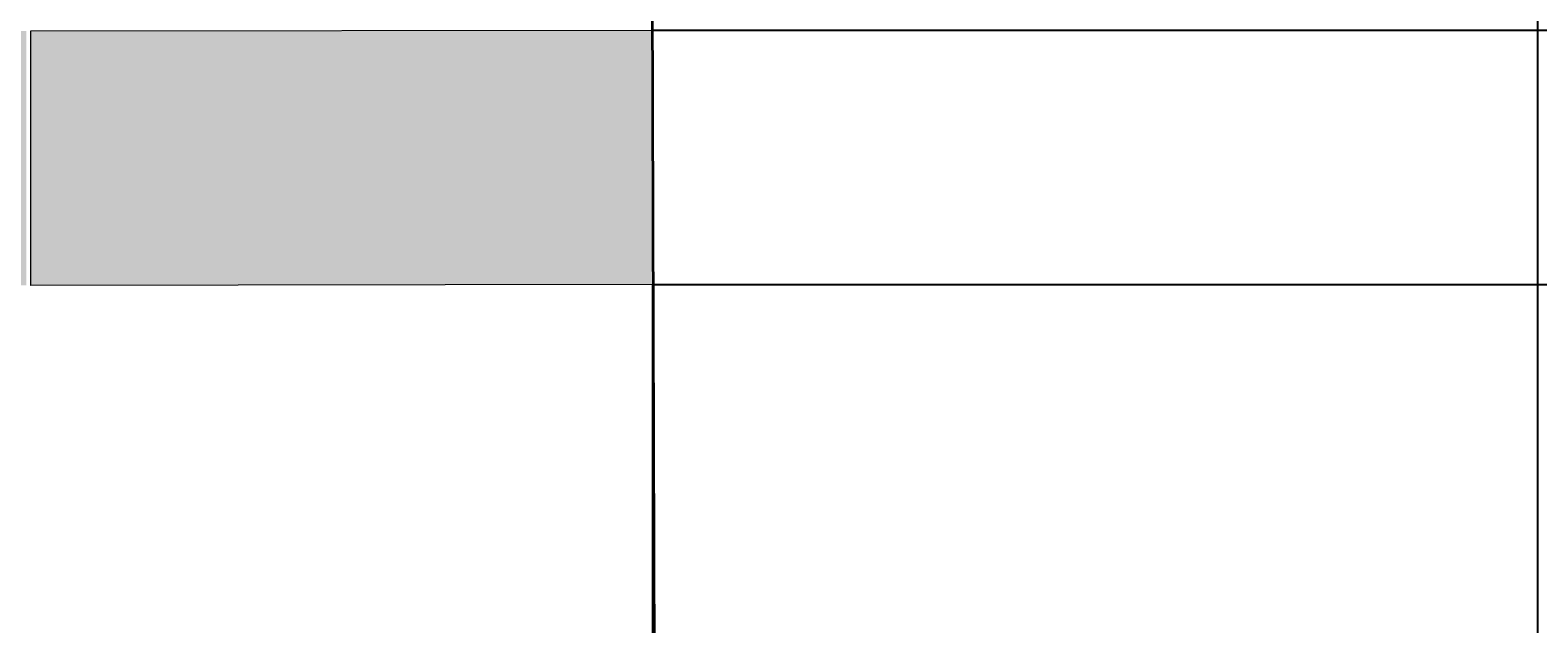
# Model space of a CAD drawing. Units: inches. Extents: x -26 to 776, y -22 to 650.
# Tile 39 of 62: x 309 to 426, y 502 to 548. Entities that reach past the tile are written whole.
import ezdxf

# ---------------------------------------------------------------- set-up
doc = ezdxf.new("R2010")
doc.units = ezdxf.units.IN
doc.header["$MEASUREMENT"] = 0
for name, color, linetype, lineweight in [('A-ANNO-DIMS', 2, 'Continuous', 18), ('A-GLAZ', 4, 'Continuous', 18), ('A-GLAZ-PATT', 9, 'Continuous', 13), ('A-WALL', 7, 'Continuous', 35)]:
    doc.layers.add(name, color=color, linetype=linetype, lineweight=lineweight)
doc.styles.get("Standard").update_dxf_attribs({"font": 'arial.ttf'})
doc.dimstyles.get("Standard").update_dxf_attribs({"dimtxt": 0.5625, "dimasz": 0.18, "dimexe": 0.18, "dimexo": 0.0625, "dimgap": 0.09, "dimtad": 0, "dimtih": 1, "dimtoh": 1, "dimdec": 4, "dimzin": 0, "dimdsep": 46, "dimlunit": 4, "dimtxsty": 'Standard', "dimcen": 0.09, "dimadec": 0, "dimazin": 0, "dimtfac": 1, "dimtdec": 4, "dimtofl": 0, "dimtmove": 0, "dimatfit": 3, "dimfxl": 1, "dimtolj": 1, "dimtzin": 0, "dimarcsym": 0})

# ---------------------------------------------------------------- blocks, each defined once
blk = doc.blocks.new('*D33')
at = {"layer": 'A-ANNO-DIMS', "color": 0, "lineweight": -2, "transparency": 16777216}
for p, q in [((357.37, 548.1), (775.34, 548.1)), ((775.16, 547.92), (775.16, 538.64)), ((775.16, 528.6), (775.16, 537.88)), ((357.37, 528.42), (775.34, 528.42))]:
    blk.add_line(p, q, dxfattribs=at)
at = {"layer": 'A-ANNO-DIMS', "color": 0, "transparency": 16777216}
for points in [[(775.13, 547.92), (775.19, 547.92), (775.16, 548.1)], [(775.13, 528.6), (775.19, 528.6), (775.16, 528.42)]]:
    blk.add_solid(points, dxfattribs=at)
at = {"layer": 'Defpoints', "color": 0, "transparency": 16777216}
for p in [(357.3, 548.1), (775.16, 548.1), (357.3, 528.42)]:
    blk.add_point(p, dxfattribs=at)
at = {"layer": 'A-ANNO-DIMS', "color": 0, "transparency": 16777216, "insert": (775.16, 538.26), "char_height": 0.562, "attachment_point": 5}
blk.add_mtext('\\A1;19.676', dxfattribs=at)
blk = doc.blocks.new('*D34')
at = {"layer": 'A-ANNO-DIMS', "color": 0, "lineweight": -2, "transparency": 16777216}
for p, q in [((228.57, 528.3), (228.57, -21.31)), ((357.3, 528.36), (357.3, -21.31)), ((228.75, -21.13), (291.71, -21.13)), ((357.12, -21.13), (294.17, -21.13))]:
    blk.add_line(p, q, dxfattribs=at)
at = {"layer": 'A-ANNO-DIMS', "color": 0, "transparency": 16777216}
for points in [[(228.75, -21.1), (228.75, -21.16), (228.57, -21.13)], [(357.12, -21.1), (357.12, -21.16), (357.3, -21.13)]]:
    blk.add_solid(points, dxfattribs=at)
at = {"layer": 'Defpoints', "color": 0, "transparency": 16777216}
for p in [(228.57, 528.36), (357.3, 528.42), (357.3, -21.13)]:
    blk.add_point(p, dxfattribs=at)
at = {"layer": 'A-ANNO-DIMS', "color": 0, "transparency": 16777216, "insert": (292.94, -21.13), "char_height": 0.562, "attachment_point": 5}
blk.add_mtext('\\A1;128.73', dxfattribs=at)
blk = doc.blocks.new('*D39')
at = {"layer": 'A-ANNO-DIMS', "color": 0, "lineweight": -2, "transparency": 16777216}
for p, q in [((289.24, 15.54), (289.24, 649.86)), ((289.42, 649.68), (356.48, 649.68)), ((425.56, 649.68), (358.51, 649.68)), ((425.74, 15.54), (425.74, 649.86))]:
    blk.add_line(p, q, dxfattribs=at)
at = {"layer": 'A-ANNO-DIMS', "color": 0, "transparency": 16777216}
for points in [[(289.42, 649.71), (289.42, 649.65), (289.24, 649.68)], [(425.56, 649.71), (425.56, 649.65), (425.74, 649.68)]]:
    blk.add_solid(points, dxfattribs=at)
at = {"layer": 'Defpoints', "color": 0, "transparency": 16777216}
for p in [(425.74, 649.68), (289.24, 15.48), (425.74, 15.48)]:
    blk.add_point(p, dxfattribs=at)
at = {"layer": 'A-ANNO-DIMS', "color": 0, "transparency": 16777216, "insert": (357.49, 649.68), "char_height": 0.562, "attachment_point": 5}
blk.add_mtext('\\A1;136.5', dxfattribs=at)

msp = doc.modelspace()

# ---------------------------------------------------------------- hatches: boundary and pattern name
at = {"layer": 'A-GLAZ-PATT'}
h = msp.add_hatch(dxfattribs=at)
h.set_pattern_fill('GOST_GLASS', color=256, scale=0.75)
h.set_pattern_definition([(45, (0, 0), (6.36396, 0), [3.75, -5.25]), (45, (1.591, 0), (6.36396, 0), [1.5, -7.5]), (45, (0, 1.591), (6.36396, 0), [1.5, -7.5])])
h.paths.add_polyline_path([(115.8402, 198.8773), (93.6448, 198.8773), (93.6448, 173.9734), (115.8402, 173.9734)])
h.paths.add_polyline_path([(144.1571, 198.8773), (115.8402, 198.8773), (115.8402, 173.9734), (144.1571, 173.9734)])
h.paths.add_polyline_path([(115.8402, 224.3396), (93.6448, 224.3396), (93.6448, 198.8773), (115.8402, 198.8773)])
h.paths.add_polyline_path([(144.1571, 248.4417), (115.8402, 248.4417), (115.8402, 224.3396), (144.1571, 224.3396)])
h.paths.add_polyline_path([(144.1571, 224.3396), (115.8402, 224.3396), (115.8402, 198.8773), (144.1571, 198.8773)])
h.paths.add_polyline_path([(170.5449, 224.3396), (144.1571, 224.3396), (144.1571, 198.8773), (170.5449, 198.8773)])
h.paths.add_polyline_path([(170.5449, 198.8773), (144.1571, 198.8773), (144.1571, 173.9734), (170.5449, 173.9734)])
h.paths.add_polyline_path([(194.6694, 198.8773), (170.5449, 198.8773), (170.5449, 173.9734), (194.6694, 173.9734)])
h.paths.add_polyline_path([(194.6694, 224.3396), (170.5449, 224.3396), (170.5449, 198.8773), (194.6694, 198.8773)])
h.paths.add_polyline_path([(194.6694, 248.4417), (170.5449, 248.4417), (170.5449, 224.3396), (194.6694, 224.3396)])
h.paths.add_polyline_path([(170.5449, 248.4417), (144.1571, 248.4417), (144.1571, 224.3396), (170.5449, 224.3396)])
h.paths.add_polyline_path([(144.1571, 269.3091), (115.8402, 269.3091), (115.8402, 248.4417), (144.1571, 248.4417)])
h.paths.add_polyline_path([(115.8402, 269.3091), (93.6448, 269.3091), (93.6448, 248.4417), (115.8402, 248.4417)])
h.paths.add_polyline_path([(115.8402, 248.4417), (93.6448, 248.4417), (93.6448, 224.3396), (115.8402, 224.3396)])
h.paths.add_polyline_path([(170.5449, 269.3091), (144.1571, 269.3091), (144.1571, 248.4417), (170.5449, 248.4417)])
h.paths.add_polyline_path([(194.6694, 269.3091), (170.5449, 269.3091), (170.5449, 248.4417), (194.6694, 248.4417)])
h.paths.add_polyline_path([(259.7413, 294.4171), (236.4647, 294.4171), (236.4647, 266.1888), (259.7413, 266.1888)])
h.paths.add_polyline_path([(285.0179, 294.4171), (261.7413, 294.4171), (261.7413, 266.1888), (285.0179, 266.1888)])
h.paths.add_polyline_path([(285.0179, 265.1888), (261.7413, 265.1888), (261.7413, 233.9172), (285.0179, 233.9172)])
h.paths.add_polyline_path([(259.7413, 265.1888), (236.4647, 265.1888), (236.4647, 233.9172), (259.7413, 233.9172)])
h.paths.add_polyline_path([(259.7413, 232.9172), (236.4647, 232.9172), (236.4647, 207.1741), (259.7413, 207.1741)])
h.paths.add_polyline_path([(285.0179, 232.9172), (261.7413, 232.9172), (261.7413, 207.1741), (285.0179, 207.1741)])
h.paths.add_polyline_path([(285.0179, 206.1741), (261.7413, 206.1741), (261.7413, 199.3298), (278.1134, 199.3298), (278.1134, 171.4173), (285.0179, 171.4173)])
h.paths.add_polyline_path([(259.7413, 206.1741), (236.4647, 206.1741), (236.4647, 199.3298), (259.7413, 199.3298)])
h.paths.add_polyline_path([(259.7413, 197.3298), (236.4647, 197.3298), (236.4647, 171.4173), (259.7413, 171.4173)])
h.paths.add_polyline_path([(276.1134, 197.3298), (261.7413, 197.3298), (261.7413, 171.4173), (276.1134, 171.4173)], flags=17)
h.paths.add_polyline_path([(255.8125, 548.0348), (228.5733, 548.0348), (228.5733, 528.3585), (255.8125, 528.3585)])
h.paths.add_polyline_path([(281.6181, 548.0348), (256.0792, 548.0348), (256.0792, 528.3585), (281.6181, 528.3585)])
h.paths.add_polyline_path([(308.8797, 548.0348), (281.789, 548.0348), (281.789, 528.3585), (308.8797, 528.3585)])
h.paths.add_polyline_path([(357.2724, 548.0995), (309.2457, 548.0348), (309.2457, 528.3585), (357.3034, 528.4233), (357.3034, 538.2614)])
h.paths.add_polyline_path([(259.7413, 437.1188), (236.4647, 437.1188), (236.4647, 408.8905), (259.7413, 408.8905)])
h.paths.add_polyline_path([(285.0179, 437.1188), (261.7413, 437.1188), (261.7413, 408.8905), (285.0179, 408.8905)])
h.paths.add_polyline_path([(259.7413, 407.8905), (236.4647, 407.8905), (236.4647, 376.6189), (259.7413, 376.6189)])
h.paths.add_polyline_path([(285.0179, 407.8905), (261.7413, 407.8905), (261.7413, 376.6189), (285.0179, 376.6189)])
h.paths.add_polyline_path([(285.0179, 375.6189), (261.7413, 375.6189), (261.7413, 349.8758), (285.0179, 349.8758)])
h.paths.add_polyline_path([(285.0179, 348.8758), (261.7413, 348.8758), (261.7413, 314.119), (285.0179, 314.119)])
h.paths.add_polyline_path([(259.7413, 348.8758), (236.4647, 348.8758), (236.4647, 314.119), (259.7413, 314.119)])
h.paths.add_polyline_path([(259.7413, 375.6189), (236.4647, 375.6189), (236.4647, 349.8758), (259.7413, 349.8758)])
h.paths.add_polyline_path([(194.6694, 404.1909), (170.5449, 404.1909), (170.5449, 383.3235), (194.6694, 383.3235)])
h.paths.add_polyline_path([(170.5449, 404.1909), (144.1571, 404.1909), (144.1571, 383.3235), (170.5449, 383.3235)])
h.paths.add_polyline_path([(144.1571, 404.1909), (115.8402, 404.1909), (115.8402, 383.3235), (144.1571, 383.3235)])
h.paths.add_polyline_path([(115.8402, 404.1909), (93.6448, 404.1909), (93.6448, 383.3235), (115.8402, 383.3235)])
h.paths.add_polyline_path([(115.8402, 383.3235), (93.6448, 383.3235), (93.6448, 359.2214), (115.8402, 359.2214)])
h.paths.add_polyline_path([(144.1571, 383.3235), (115.8402, 383.3235), (115.8402, 359.2214), (144.1571, 359.2214)])
h.paths.add_polyline_path([(115.8402, 359.2214), (93.6448, 359.2214), (93.6448, 333.7591), (115.8402, 333.7591)])
h.paths.add_polyline_path([(144.1571, 359.2214), (115.8402, 359.2214), (115.8402, 333.7591), (144.1571, 333.7591)])
h.paths.add_polyline_path([(115.8402, 333.7591), (93.6448, 333.7591), (93.6448, 308.8552), (115.8402, 308.8552)])
h.paths.add_polyline_path([(144.1571, 333.7591), (115.8402, 333.7591), (115.8402, 308.8552), (144.1571, 308.8552)])
h.paths.add_polyline_path([(170.5449, 333.7591), (144.1571, 333.7591), (144.1571, 308.8552), (170.5449, 308.8552)])
h.paths.add_polyline_path([(170.5449, 359.2214), (144.1571, 359.2214), (144.1571, 333.7591), (170.5449, 333.7591)])
h.paths.add_polyline_path([(170.5449, 383.3235), (144.1571, 383.3235), (144.1571, 359.2214), (170.5449, 359.2214)])
h.paths.add_polyline_path([(194.6694, 383.3235), (170.5449, 383.3235), (170.5449, 359.2214), (194.6694, 359.2214)])
h.paths.add_polyline_path([(194.6694, 359.2214), (170.5449, 359.2214), (170.5449, 333.7591), (194.6694, 333.7591)])
h.paths.add_polyline_path([(194.6694, 333.7591), (170.5449, 333.7591), (170.5449, 308.8552), (194.6694, 308.8552)])

# ---------------------------------------------------------------- linework, layer by layer
at = {"layer": 'A-GLAZ'}
msp.add_lwpolyline([(309.2457, 548.0348), (357.3034, 548.0996), (357.3034, 528.4233), (309.2457, 528.3585)], close=True, dxfattribs=at)
at = {"layer": 'A-WALL'}
msp.add_line((357.0669, 613.2713), (357.4929, 478.1838), dxfattribs=at)

# ---------------------------------------------------------------- dimensions: what is measured, and where the dimension line sits
at = {"layer": 'A-ANNO-DIMS'}
for base, p1, p2, override, picture, middle in [((425.7434, 649.6763), (289.2424, 15.4824), (425.7434, 15.4824), {"dimdec": 1, "dimlfac": 1, "dimrnd": 0, "dimzin": 0, "dimdsep": 46, "dimlunit": 2}, '*D39', (357.4929, 649.6763)), ((357.3034, -21.1349), (228.5733, 528.3585), (357.3034, 528.4233), {"dimdec": 2, "dimlfac": 1, "dimrnd": 0, "dimzin": 0, "dimdsep": 46, "dimlunit": 2}, '*D34', (292.9384, -21.1349))]:
    dim = msp.add_linear_dim(base=base, p1=p1, p2=p2, dimstyle='Standard', override=override, dxfattribs=at)
    dim.commit()
    dim.dimension.update_dxf_attribs({"geometry": picture, "text_midpoint": middle})
dim = msp.add_linear_dim(base=(775.1553, 548.0996), p1=(357.3034, 528.4233), p2=(357.3034, 548.0996), angle=90, dimstyle='Standard', override={"dimdec": 3, "dimlfac": 1, "dimrnd": 0, "dimzin": 0, "dimdsep": 46, "dimlunit": 2}, dxfattribs=at)
dim.commit()
dim.dimension.update_dxf_attribs({"geometry": '*D33', "text_midpoint": (775.1553, 538.2614)})

doc.saveas('drawing.dxf')
